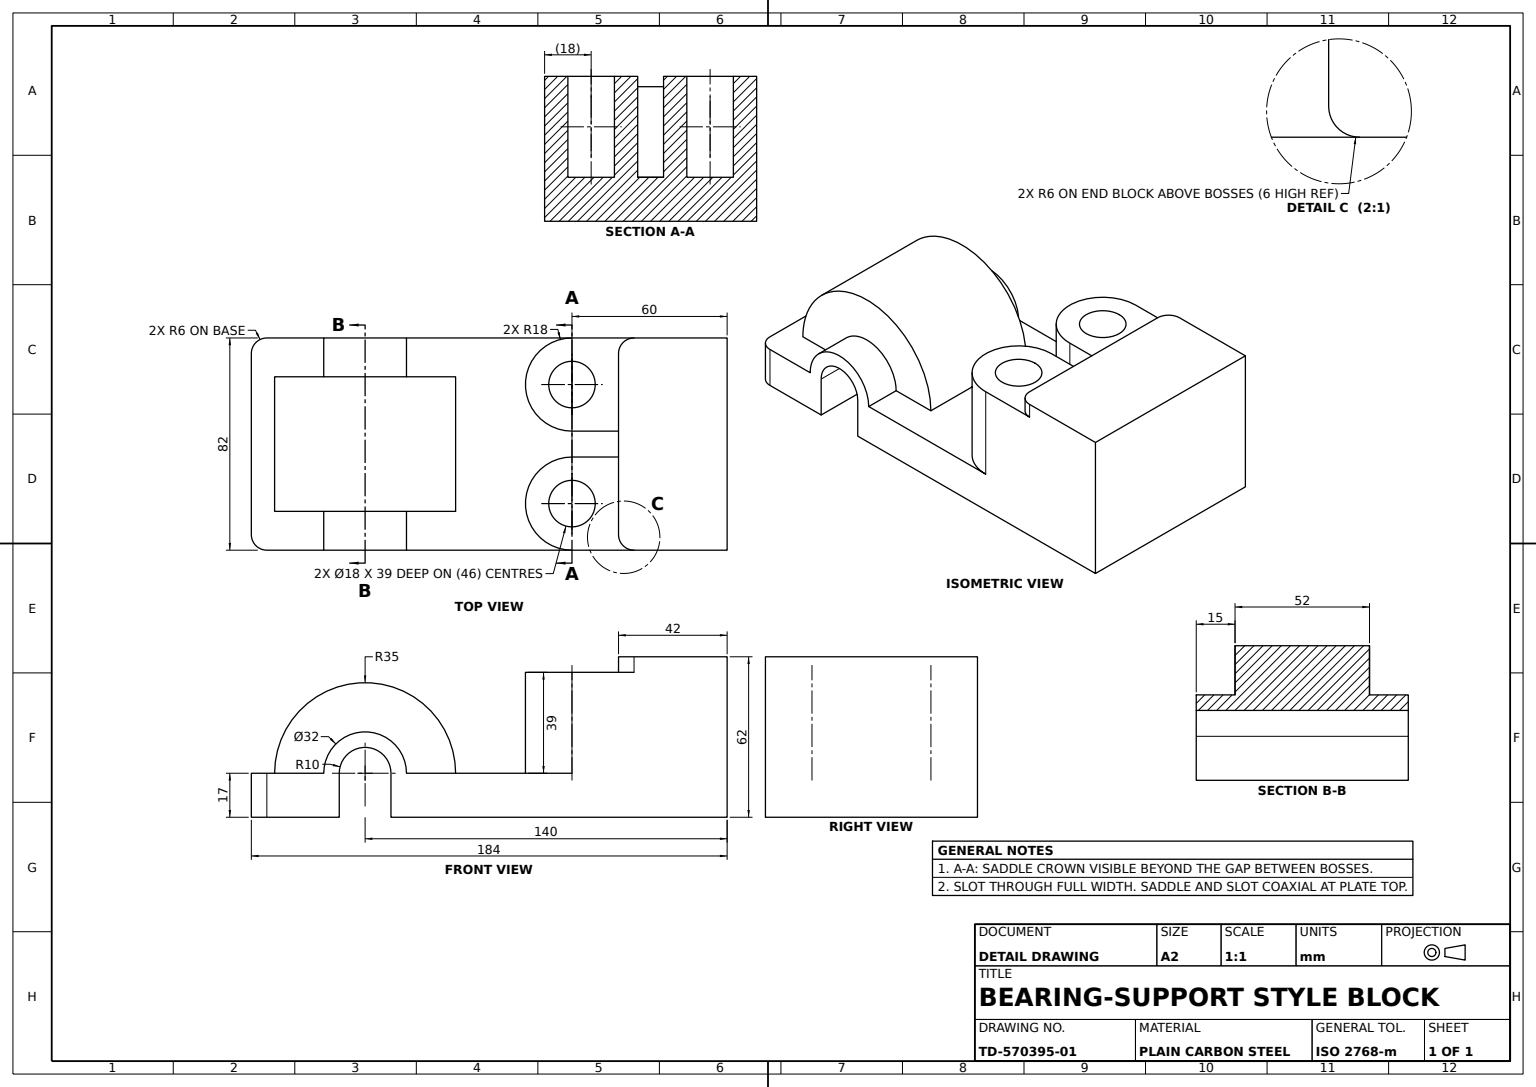
from build123d import *

# Parameters (mm, degrees)
BASE_PLATE_184X82X17_DEPTH      = 17
BEARING_SADDLE_DEPTH            = 45
RAISED_PAD_DEPTH                = 82
STEP_PROFILE_DEPTH              = 82
SLOT_CUT_DEPTH                  = 82
BOLT_BOSSES_SKETCH_R            = 9
BOLT_BOSSES_2X_WITH_HOLES_DEPTH = 39
END_BLOCK_DEPTH                 = 26


with BuildPart() as part:
    # Base Plate Sketch → Base Plate 184x82x17 (new body)
    with BuildSketch(Plane(origin=(0, 0, 0), x_dir=(1, 0, 0), z_dir=(0, 1, 0))):
        with BuildLine():
            Line((-86, -41), (92, -41))
            Line((92, -41), (92, 41))
            Line((92, 41), (-86, 41))
            ThreePointArc((-86, 41), (-90.242640687, 39.242640687), (-92, 35))
            Line((-92, 35), (-92, -35))
            ThreePointArc((-92, -35), (-90.242640687, -39.242640687), (-86, -41))
        make_face()
    extrude(amount=BASE_PLATE_184X82X17_DEPTH)

    # Bearing Saddle Sketch → Bearing Saddle (add)
    with BuildSketch(Plane(origin=(0, 17, 0), x_dir=(1, 0, 0), z_dir=(0, 1, 0))):
        with BuildLine():
            Line((92, -41), (56, -41))
            ThreePointArc((56, -41), (51.757359313, -39.242640687), (50, -35))
            Line((50, -35), (50, 35))
            ThreePointArc((50, 35), (51.757359313, 39.242640687), (56, 41))
            Line((56, 41), (92, 41))
            Line((92, 41), (92, -41))
        make_face()
    extrude(amount=BEARING_SADDLE_DEPTH)

    # Raised Pad Sketch → Raised Pad (add)
    with BuildSketch(Plane.XY.offset(41)):
        with BuildLine():
            Line((-58, 17), (-58, 0))
            Line((-58, 0), (-38, 0))
            Line((-38, 0), (-38, 17))
            ThreePointArc((-38, 17), (-48, 27), (-58, 17))
        make_face()
    extrude(amount=-RAISED_PAD_DEPTH)

    # Step Profile Sketch → Step Profile (add)
    with BuildSketch(Plane.XY.offset(41)):
        with BuildLine():
            Line((-64, 17), (-58, 17))
            ThreePointArc((-58, 17), (-48, 27), (-38, 17))
            Line((-38, 17), (-32, 17))
            ThreePointArc((-32, 17), (-48, 33), (-64, 17))
        make_face()
    extrude(amount=-STEP_PROFILE_DEPTH)

    # Slot Cut Sketch → Slot Cut (cut)
    with BuildSketch(Plane.XY.offset(41)):
        with BuildLine():
            Line((-58, 17), (-58, 0))
            Line((-58, 0), (-38, 0))
            Line((-38, 0), (-38, 17))
            ThreePointArc((-38, 17), (-48, 27), (-58, 17))
        make_face()
    extrude(amount=-SLOT_CUT_DEPTH, mode=Mode.SUBTRACT)

    # Bolt Bosses Sketch → Bolt Bosses 2x with Holes (add)
    # profile 1 of 2: a face of its own
    with BuildSketch(Plane(origin=(0, 17, 0), x_dir=(1, 0, 0), z_dir=(0, 1, 0))):
        with BuildLine():
            Line((32, 41), (56, 41))
            Line((56, 41), (56, 5))
            Line((56, 5), (32, 5))
            ThreePointArc((32, 5), (14, 23), (32, 41))
        make_face()
        with Locations(Location((32, 23, 0), (0, 0, 270))):
            Circle(BOLT_BOSSES_SKETCH_R, mode=Mode.SUBTRACT)
    # profile 2 of 2: a face of its own
    with BuildSketch(Plane(origin=(0, 17, 0), x_dir=(1, 0, 0), z_dir=(0, 1, 0))):
        with BuildLine():
            Line((32, -5), (56, -5))
            Line((56, -5), (56, -41))
            Line((56, -41), (32, -41))
            ThreePointArc((32, -41), (14, -23), (32, -5))
        make_face()
        with Locations(Location((32, -23, 0), (0, 0, 270))):
            Circle(BOLT_BOSSES_SKETCH_R, mode=Mode.SUBTRACT)
    extrude(amount=BOLT_BOSSES_2X_WITH_HOLES_DEPTH)

    # End Block Sketch → End Block (add, symmetric)
    with BuildSketch(Plane.XY):
        with BuildLine():
            Line((-83, 17), (-64, 17))
            ThreePointArc((-64, 17), (-48, 33), (-32, 17))
            Line((-32, 17), (-13, 17))
            ThreePointArc((-13, 17), (-48, 52), (-83, 17))
        make_face()
    extrude(amount=END_BLOCK_DEPTH, both=True)


solid = part.part
